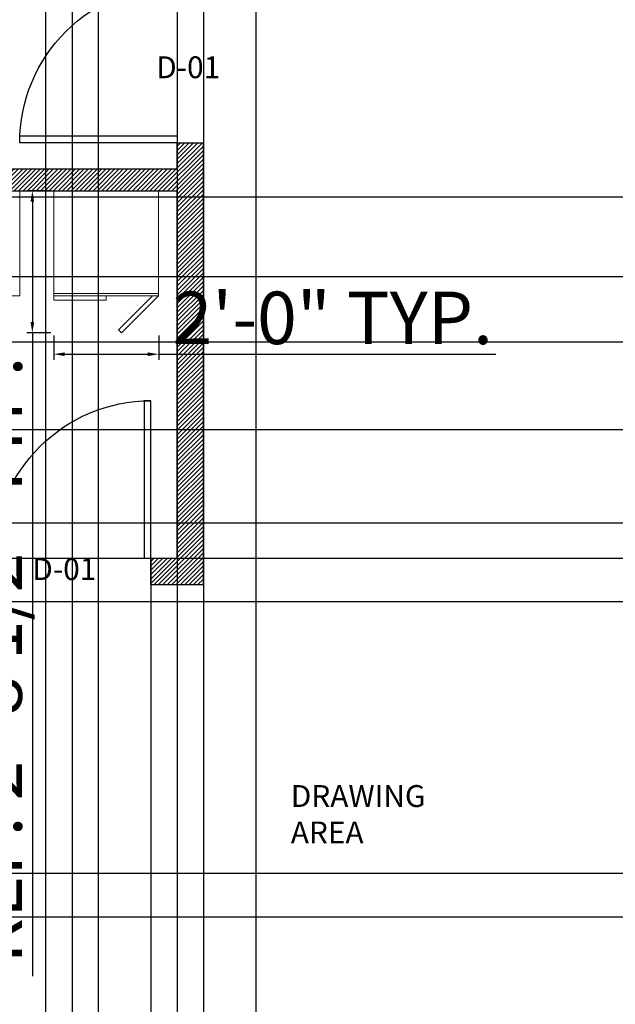
# Model space of a CAD drawing. Units: inches. Extents: x 2386 to 3029, y 792 to 1465.
# Tile 9 of 12: x 2588 to 2724, y 1044 to 1269. Entities that reach past the tile are written whole.
import ezdxf

# ---------------------------------------------------------------- set-up
doc = ezdxf.new("R2010")
doc.units = ezdxf.units.IN
for name, color, linetype, lineweight in [('A-AREA-IDEN', 4, 'Continuous', 25), ('A-DIMS', 1, 'Continuous', 18), ('A-DOOR', 2, 'Continuous', 25), ('A-EQPM', 8, 'Continuous', 18), ('A-FLOR-CASE', 6, 'Continuous', 18), ('A-TEXT', 4, 'Continuous', 25), ('A-WALL-INT', 9, 'Continuous', 30), ('A-WALL-PATT', 9, 'Continuous', 13)]:
    doc.layers.add(name, color=color, linetype=linetype, lineweight=lineweight)
doc.styles.get("Standard").update_dxf_attribs({"font": 'arial.ttf'})
doc.dimstyles.new('ISO-25', dxfattribs={"dimtxt": 12, "dimasz": 2.5, "dimexe": 1.25, "dimexo": 0.625, "dimtad": 1, "dimlunit": 4, "dimtxsty": 'Standard', "dimcen": 2.5, "dimadec": 0, "dimazin": 0, "dimtfac": 1, "dimtmove": 0, "dimatfit": 3, "dimfxl": 1, "dimarcsym": 0})

# ---------------------------------------------------------------- blocks, each defined once
blk = doc.blocks.new('*U13')
for p, q in [((0, 0), (0, 6)), ((40, 0), (40, 6))]:
    blk.add_line(p, q)
blk.add_lwpolyline([(0, 0), (0, -40), (1.75, -40), (1.75, 0)], close=True)
blk.add_arc((0, 0), 40, 270, 0)
blk = doc.blocks.new('*U14')
for p, q in [((-40, 0), (-40, 6)), ((0, 0), (0, 6))]:
    blk.add_line(p, q)
blk.add_lwpolyline([(0, 0), (0, -40), (-1.75, -40), (-1.75, 0)], close=True)
blk.add_arc((0, 0), 40, 180, 270)
blk = doc.blocks.new('REFRIGERATOR-24')
blk.add_line((23.5, 24), (23.5, 0))
for points in [[(24, 0), (0, 0), (0, 24), (24, 24)], [(24, 22.59), (31.78, 14.81), (32.49, 15.51), (24, 24), (24, 0), (25, 0), (25, 12), (24, 12)]]:
    blk.add_lwpolyline(points)
blk = doc.blocks.new('*D52')
at = {"layer": 'A-DIMS', "color": 0, "lineweight": -2, "transparency": 16777216}
for p, q in [((2595.33, 1229.95), (2589.83, 1229.95)), ((2591.08, 1227.45), (2591.08, 1199.96)), ((2595.33, 1197.46), (2589.83, 1197.46)), ((2591.08, 1197.46), (2591.08, 1050.38))]:
    blk.add_line(p, q, dxfattribs=at)
at = {"layer": 'A-DIMS', "color": 0, "transparency": 16777216}
for points in [[(2590.67, 1227.45), (2591.5, 1227.45), (2591.08, 1229.95)], [(2590.67, 1199.96), (2591.5, 1199.96), (2591.08, 1197.46)]]:
    blk.add_solid(points, dxfattribs=at)
at = {"layer": 'Defpoints', "color": 0, "transparency": 16777216}
for p in [(2595.96, 1229.95), (2591.08, 1197.46), (2595.96, 1197.46)]:
    blk.add_point(p, dxfattribs=at)
at = {"layer": 'A-DIMS', "color": 0, "transparency": 16777216, "insert": (2584.25, 1122.67), "char_height": 12, "attachment_point": 5, "rotation": 90}
blk.add_mtext('REF. 2\'-8 1/2" TYP.', dxfattribs=at)
blk = doc.blocks.new('*D53')
at = {"layer": 'A-DIMS', "color": 0, "lineweight": -2, "transparency": 16777216}
for p, q in [((2595.96, 1196.84), (2595.96, 1191.34)), ((2619.96, 1196.84), (2619.96, 1191.34)), ((2598.46, 1192.59), (2617.46, 1192.59)), ((2619.96, 1192.59), (2697.06, 1192.59))]:
    blk.add_line(p, q, dxfattribs=at)
at = {"layer": 'A-DIMS', "color": 0, "transparency": 16777216}
for points in [[(2598.46, 1193.01), (2598.46, 1192.17), (2595.96, 1192.59)], [(2617.46, 1193.01), (2617.46, 1192.17), (2619.96, 1192.59)]]:
    blk.add_solid(points, dxfattribs=at)
at = {"layer": 'Defpoints', "color": 0, "transparency": 16777216}
for p in [(2595.96, 1197.46), (2619.96, 1197.46), (2619.96, 1192.59)]:
    blk.add_point(p, dxfattribs=at)
at = {"layer": 'A-DIMS', "color": 0, "transparency": 16777216, "insert": (2659.76, 1199.34), "char_height": 12, "attachment_point": 5}
blk.add_mtext('2\'-0" TYP.', dxfattribs=at)
blk = doc.blocks.new('*D66')
at = {"layer": 'A-DIMS', "color": 0, "lineweight": -2, "transparency": 16777216}
for p, q in [((2630.19, 1378.32), (2630.19, 808)), ((2642.19, 1378.32), (2642.19, 808)), ((2632.69, 809.25), (2639.69, 809.25)), ((2642.19, 809.25), (2676.71, 809.25))]:
    blk.add_line(p, q, dxfattribs=at)
at = {"layer": 'A-DIMS', "color": 0, "transparency": 16777216}
for points in [[(2632.69, 809.66), (2632.69, 808.83), (2630.19, 809.25)], [(2639.69, 809.66), (2639.69, 808.83), (2642.19, 809.25)]]:
    blk.add_solid(points, dxfattribs=at)
at = {"layer": 'Defpoints', "color": 0, "transparency": 16777216}
for p in [(2630.19, 1378.95), (2642.19, 1378.95), (2642.19, 809.25)]:
    blk.add_point(p, dxfattribs=at)
at = {"layer": 'A-DIMS', "color": 0, "transparency": 16777216, "insert": (2660.7, 816), "char_height": 12, "attachment_point": 5}
blk.add_mtext('1\'-0"', dxfattribs=at)
blk = doc.blocks.new('*D75')
at = {"layer": 'A-DIMS', "color": 0, "lineweight": -2, "transparency": 16777216}
for p, q in [((2929.89, 1195.39), (2929.89, 1229.91)), ((2498.82, 1195.39), (2931.14, 1195.39)), ((2929.89, 1177.89), (2929.89, 1192.89)), ((2498.82, 1175.39), (2931.14, 1175.39))]:
    blk.add_line(p, q, dxfattribs=at)
at = {"layer": 'A-DIMS', "color": 0, "transparency": 16777216}
for points in [[(2929.47, 1192.89), (2930.31, 1192.89), (2929.89, 1195.39)], [(2929.47, 1177.89), (2930.31, 1177.89), (2929.89, 1175.39)]]:
    blk.add_solid(points, dxfattribs=at)
at = {"layer": 'Defpoints', "color": 0, "transparency": 16777216}
for p in [(2498.19, 1195.39), (2929.89, 1195.39), (2498.19, 1175.39)]:
    blk.add_point(p, dxfattribs=at)
at = {"layer": 'A-DIMS', "color": 0, "transparency": 16777216, "insert": (2923.14, 1213.9), "char_height": 12, "attachment_point": 5, "rotation": 90}
blk.add_mtext('1\'-8"', dxfattribs=at)
blk = doc.blocks.new('*D79')
at = {"layer": 'A-DIMS', "color": 0, "lineweight": -2, "transparency": 16777216}
for p, q in [((2929.89, 1073.95), (2929.89, 1118.92)), ((2516.82, 1073.95), (2931.14, 1073.95)), ((2929.89, 1066.45), (2929.89, 1071.45)), ((2516.82, 1063.95), (2931.14, 1063.95))]:
    blk.add_line(p, q, dxfattribs=at)
at = {"layer": 'A-DIMS', "color": 0, "transparency": 16777216}
for points in [[(2929.47, 1071.45), (2930.31, 1071.45), (2929.89, 1073.95)], [(2929.47, 1066.45), (2930.31, 1066.45), (2929.89, 1063.95)]]:
    blk.add_solid(points, dxfattribs=at)
at = {"layer": 'Defpoints', "color": 0, "transparency": 16777216}
for p in [(2516.19, 1073.95), (2929.89, 1073.95), (2516.19, 1063.95)]:
    blk.add_point(p, dxfattribs=at)
at = {"layer": 'A-DIMS', "color": 0, "transparency": 16777216, "insert": (2923.14, 1097.68), "char_height": 12, "attachment_point": 5, "rotation": 90}
blk.add_mtext('0\'-10"', dxfattribs=at)
blk = doc.blocks.new('*D81')
at = {"layer": 'A-DIMS', "color": 0, "lineweight": -2, "transparency": 16777216}
for p, q in [((2432.49, 1153.95), (2432.49, 1188.47)), ((2809.57, 1153.95), (2431.24, 1153.95)), ((2432.49, 1138.45), (2432.49, 1151.45)), ((2809.57, 1135.95), (2431.24, 1135.95))]:
    blk.add_line(p, q, dxfattribs=at)
at = {"layer": 'A-DIMS', "color": 0, "transparency": 16777216}
for points in [[(2432.07, 1151.45), (2432.91, 1151.45), (2432.49, 1153.95)], [(2432.07, 1138.45), (2432.91, 1138.45), (2432.49, 1135.95)]]:
    blk.add_solid(points, dxfattribs=at)
at = {"layer": 'Defpoints', "color": 0, "transparency": 16777216}
for p in [(2432.49, 1153.95), (2810.19, 1153.95), (2810.19, 1135.95)]:
    blk.add_point(p, dxfattribs=at)
at = {"layer": 'A-DIMS', "color": 0, "transparency": 16777216, "insert": (2425.74, 1172.46), "char_height": 12, "attachment_point": 5, "rotation": 90}
blk.add_mtext('1\'-6"', dxfattribs=at)
blk = doc.blocks.new('*D82')
at = {"layer": 'A-DIMS', "color": 0, "lineweight": -2, "transparency": 16777216}
for p, q in [((2600.19, 1306.32), (2600.19, 808)), ((2624.19, 1306.32), (2624.19, 808)), ((2602.69, 809.25), (2621.69, 809.25)), ((2624.19, 809.25), (2660.04, 809.25))]:
    blk.add_line(p, q, dxfattribs=at)
at = {"layer": 'A-DIMS', "color": 0, "transparency": 16777216}
for points in [[(2602.69, 809.66), (2602.69, 808.83), (2600.19, 809.25)], [(2621.69, 809.66), (2621.69, 808.83), (2624.19, 809.25)]]:
    blk.add_solid(points, dxfattribs=at)
at = {"layer": 'Defpoints', "color": 0, "transparency": 16777216}
for p in [(2600.19, 1306.95), (2624.19, 1306.95), (2624.19, 809.25)]:
    blk.add_point(p, dxfattribs=at)
at = {"layer": 'A-DIMS', "color": 0, "transparency": 16777216, "insert": (2643.37, 816), "char_height": 12, "attachment_point": 5}
blk.add_mtext('2\'-0"', dxfattribs=at)
blk = doc.blocks.new('*D87')
at = {"layer": 'A-DIMS', "color": 0, "lineweight": -2, "transparency": 16777216}
for p, q in [((2594.19, 921.57), (2594.19, 1427.9)), ((2606.19, 921.57), (2606.19, 1427.9)), ((2596.69, 1426.65), (2603.69, 1426.65)), ((2606.19, 1426.65), (2640.71, 1426.65))]:
    blk.add_line(p, q, dxfattribs=at)
at = {"layer": 'A-DIMS', "color": 0, "transparency": 16777216}
for points in [[(2596.69, 1427.06), (2596.69, 1426.23), (2594.19, 1426.65)], [(2603.69, 1427.06), (2603.69, 1426.23), (2606.19, 1426.65)]]:
    blk.add_solid(points, dxfattribs=at)
at = {"layer": 'Defpoints', "color": 0, "transparency": 16777216}
for p in [(2606.19, 1426.65), (2594.19, 920.95), (2606.19, 920.95)]:
    blk.add_point(p, dxfattribs=at)
at = {"layer": 'A-DIMS', "color": 0, "transparency": 16777216, "insert": (2624.7, 1433.4), "char_height": 12, "attachment_point": 5}
blk.add_mtext('1\'-0"', dxfattribs=at)
blk = doc.blocks.new('*D92')
at = {"layer": 'A-DIMS', "color": 0, "lineweight": -2, "transparency": 16777216}
for p, q in [((2618.19, 1145.32), (2618.19, 808)), ((2624.19, 1145.32), (2624.19, 808)), ((2615.69, 809.25), (2613.19, 809.25)), ((2618.19, 809.25), (2624.19, 809.25)), ((2626.69, 809.25), (2662.34, 809.25))]:
    blk.add_line(p, q, dxfattribs=at)
at = {"layer": 'A-DIMS', "color": 0, "transparency": 16777216}
for points in [[(2615.69, 809.66), (2615.69, 808.83), (2618.19, 809.25)], [(2626.69, 809.66), (2626.69, 808.83), (2624.19, 809.25)]]:
    blk.add_solid(points, dxfattribs=at)
at = {"layer": 'Defpoints', "color": 0, "transparency": 16777216}
for p in [(2618.19, 1145.95), (2624.19, 1145.95), (2624.19, 809.25)]:
    blk.add_point(p, dxfattribs=at)
at = {"layer": 'A-DIMS', "color": 0, "transparency": 16777216, "insert": (2645.76, 816), "char_height": 12, "attachment_point": 5}
blk.add_mtext('0\'-6"', dxfattribs=at)
blk = doc.blocks.new('*D99')
at = {"layer": 'A-DIMS', "color": 0, "lineweight": -2, "transparency": 16777216}
for p, q in [((2530.41, 1210.29), (2530.41, 808)), ((2563.26, 1210.63), (2563.26, 808)), ((2532.91, 809.25), (2560.76, 809.25)), ((2563.26, 809.25), (2599.11, 809.25))]:
    blk.add_line(p, q, dxfattribs=at)
at = {"layer": 'A-DIMS', "color": 0, "transparency": 16777216}
for points in [[(2532.91, 809.66), (2532.91, 808.83), (2530.41, 809.25)], [(2560.76, 809.66), (2560.76, 808.83), (2563.26, 809.25)]]:
    blk.add_solid(points, dxfattribs=at)
at = {"layer": 'Defpoints', "color": 0, "transparency": 16777216}
for p in [(2563.26, 1211.26), (2530.41, 1210.91), (2563.26, 809.25)]:
    blk.add_point(p, dxfattribs=at)
at = {"layer": 'A-DIMS', "color": 0, "transparency": 16777216, "insert": (2582.43, 816), "char_height": 12, "attachment_point": 5}
blk.add_mtext('2\'-9"', dxfattribs=at)
blk = doc.blocks.new('*D100')
at = {"layer": 'A-DIMS', "color": 0, "lineweight": -2, "transparency": 16777216}
for p, q in [((2562.86, 1228.59), (2931.14, 1228.59)), ((2929.89, 1226.09), (2929.89, 1212.84)), ((2563.05, 1210.34), (2931.14, 1210.34)), ((2929.89, 1210.34), (2929.89, 1147.86))]:
    blk.add_line(p, q, dxfattribs=at)
at = {"layer": 'A-DIMS', "color": 0, "transparency": 16777216}
for points in [[(2929.47, 1226.09), (2930.31, 1226.09), (2929.89, 1228.59)], [(2929.47, 1212.84), (2930.31, 1212.84), (2929.89, 1210.34)]]:
    blk.add_solid(points, dxfattribs=at)
at = {"layer": 'Defpoints', "color": 0, "transparency": 16777216}
for p in [(2562.24, 1228.59), (2562.43, 1210.34), (2929.89, 1210.34)]:
    blk.add_point(p, dxfattribs=at)
at = {"layer": 'A-DIMS', "color": 0, "transparency": 16777216, "insert": (2923.06, 1177.85), "char_height": 12, "attachment_point": 5, "rotation": 90}
blk.add_mtext('1\'-6 1/2"', dxfattribs=at)
blk = doc.blocks.new('*D101')
at = {"layer": 'A-DIMS', "color": 0, "lineweight": -2, "transparency": 16777216}
for p, q in [((2929.89, 1175.39), (2929.89, 1239.21)), ((2480.82, 1175.39), (2931.14, 1175.39)), ((2929.89, 1148.45), (2929.89, 1172.89)), ((2480.82, 1145.95), (2931.14, 1145.95))]:
    blk.add_line(p, q, dxfattribs=at)
at = {"layer": 'A-DIMS', "color": 0, "transparency": 16777216}
for points in [[(2929.47, 1172.89), (2930.31, 1172.89), (2929.89, 1175.39)], [(2929.47, 1148.45), (2930.31, 1148.45), (2929.89, 1145.95)]]:
    blk.add_solid(points, dxfattribs=at)
at = {"layer": 'Defpoints', "color": 0, "transparency": 16777216}
for p in [(2480.19, 1175.39), (2929.89, 1175.39), (2480.19, 1145.95)]:
    blk.add_point(p, dxfattribs=at)
at = {"layer": 'A-DIMS', "color": 0, "transparency": 16777216, "insert": (2923.06, 1208.55), "char_height": 12, "attachment_point": 5, "rotation": 90}
blk.add_mtext('2\'-5 1/2"', dxfattribs=at)

msp = doc.modelspace()

# ---------------------------------------------------------------- hatches: boundary and pattern name
at = {"layer": 'A-WALL-PATT'}
h = msp.add_hatch(dxfattribs=at)
h.set_pattern_fill('JIS_WOOD', color=256)
h.paths.add_polyline_path([(2624.19, 1229.948), (2624.19, 1145.948), (2618.19, 1145.948), (2618.19, 1140.548), (2618.19, 1139.948), (2630.19, 1139.948), (2630.19, 1240.948), (2624.19, 1240.948), (2624.19, 1234.948), (2480.19, 1234.948), (2480.19, 1229.948)])
h.paths.add_polyline_path([(2582.19, 1139.948), (2582.19, 1145.948), (2480.19, 1145.948), (2480.19, 1139.948)], flags=17)
h.paths.add_polyline_path([(2480.19, 1007.948), (2480.19, 1001.948), (2546.19, 1001.948), (2546.19, 1007.348), (2546.19, 1007.948)])
h.paths.add_polyline_path([(2594.19, 1007.948), (2582.19, 1007.948), (2582.19, 1001.948), (2588.19, 1001.948), (2588.19, 856.948), (2594.19, 856.948), (2594.19, 914.948), (2606.19, 914.948), (2606.19, 920.948), (2594.19, 920.948)])
h.paths.add_polyline_path([(2738.19, 1015.948), (2882.19, 1015.948), (2882.19, 1021.948), (2738.19, 1021.948), (2738.19, 1111.948), (2732.19, 1111.948), (2732.19, 920.948), (2720.19, 920.948), (2720.19, 914.948), (2732.19, 914.948), (2732.19, 856.948), (2738.19, 856.948)])
h.paths.add_polyline_path([(2660.19, 914.948), (2660.19, 920.948), (2648.19, 920.948), (2648.19, 914.948)])
h.paths.add_polyline_path([(2738.19, 1159.948), (2738.19, 1165.948), (2737.59, 1165.948), (2732.19, 1165.948), (2732.19, 1147.948), (2737.59, 1147.948), (2738.19, 1147.948), (2738.19, 1153.948), (2882.19, 1153.948), (2882.19, 1159.948)])
h.paths.add_polyline_path([(2732.19, 1201.948), (2738.19, 1201.948), (2738.19, 1303.948), (2774.19, 1303.948), (2774.19, 1308.948), (2768.19, 1308.948), (2768.19, 1378.948), (2762.19, 1378.948), (2762.19, 1308.948), (2726.19, 1308.948), (2726.19, 1303.948), (2732.19, 1303.948)])
h.paths.add_polyline_path([(2696.19, 1303.948), (2696.19, 1308.948), (2630.19, 1308.948), (2630.19, 1378.948), (2624.19, 1378.948), (2624.19, 1276.948), (2630.19, 1276.948), (2630.19, 1303.948)])

# ---------------------------------------------------------------- linework, layer by layer
at = {"layer": 'A-FLOR-CASE'}
msp.add_lwpolyline([(2504.19, 1145.948), (2504.19, 1205.948), (2588.19, 1205.948), (2588.19, 1229.948)], dxfattribs=at)
at = {"layer": 'A-WALL-INT'}
for p, q in [((2624.19, 1234.948), (2624.19, 1240.948)), ((2624.19, 1240.948), (2630.19, 1240.948)), ((2630.19, 1139.948), (2630.19, 1240.948)), ((2480.19, 1234.948), (2624.19, 1234.948)), ((2480.19, 1229.948), (2624.19, 1229.948)), ((2624.19, 1145.948), (2624.19, 1229.948)), ((2618.19, 1139.948), (2618.19, 1145.948)), ((2618.19, 1145.948), (2624.19, 1145.948)), ((2618.19, 1139.948), (2630.19, 1139.948))]:
    msp.add_line(p, q, dxfattribs=at)

# ---------------------------------------------------------------- block references
at = {"layer": 'A-DOOR', "xscale": -0.9, "yscale": 0.9, "zscale": 0.9}
for name, p, rotation in [('*U13', (2624.19, 1240.948), 270), ('*U14', (2618.19, 1145.948), 180)]:
    msp.add_blockref(name, p, dxfattribs=dict(at, rotation=rotation))
at = {"layer": 'A-EQPM', "rotation": 269.9999999999993}
msp.add_blockref('REFRIGERATOR-24', (2595.956, 1229.948), dxfattribs=at)

# ---------------------------------------------------------------- texts
at = {"layer": 'A-AREA-IDEN', "insert": (2650.166, 1094.069), "char_height": 5, "attachment_point": 1}
msp.add_mtext_dynamic_manual_height_columns('DRAWING    AREA', width=38.22215, gutter_width=12.5, heights=[0], dxfattribs=at)
at = {"layer": 'A-TEXT', "char_height": 5, "attachment_point": 1}
for insert in [(2619.392, 1260.698), (2591.074, 1145.947)]:
    msp.add_mtext_dynamic_manual_height_columns('D-01', width=38.22215, gutter_width=12.5, heights=[0], dxfattribs=dict(at, insert=insert))

# ---------------------------------------------------------------- dimensions: what is measured, and where the dimension line sits
at = {"layer": 'A-DIMS'}
for base, p1, p2, picture, middle in [((2606.19, 1426.648), (2594.19, 920.948), (2606.19, 920.948), '*D87', (2624.7, 1433.4)), ((2642.19, 809.248), (2630.19, 1378.948), (2642.19, 1378.948), '*D66', (2660.7, 816)), ((2624.19, 809.248), (2600.19, 1306.948), (2624.19, 1306.948), '*D82', (2643.367, 816)), ((2563.257, 809.248), (2530.413, 1210.915), (2563.257, 1211.257), '*D99', (2582.434, 816)), ((2624.19, 809.248), (2618.19, 1145.948), (2624.19, 1145.948), '*D92', (2645.765, 816))]:
    dim = msp.add_linear_dim(base=base, p1=p1, p2=p2, dimstyle='ISO-25', override={"dimdec": 1, "dimlfac": 1, "dimrnd": 0, "dimzin": 1, "dimdsep": 46, "dimlunit": 4, "dimfrac": 2}, dxfattribs=at)
    dim.commit()
    dim.dimension.update_dxf_attribs({"geometry": picture, "text_midpoint": middle})
for base, p1, p2, picture, middle in [((2929.89, 1175.392), (2480.19, 1145.948), (2480.19, 1175.392), '*D101', (2923.06, 1208.55)), ((2929.89, 1195.392), (2498.19, 1175.392), (2498.19, 1195.392), '*D75', (2923.138, 1213.902)), ((2929.89, 1210.342), (2562.236, 1228.595), (2562.425, 1210.342), '*D100', (2923.06, 1177.852)), ((2432.49, 1153.948), (2810.19, 1135.948), (2810.19, 1153.948), '*D81', (2425.738, 1172.458)), ((2929.89, 1073.948), (2516.19, 1063.948), (2516.19, 1073.948), '*D79', (2923.138, 1097.684))]:
    dim = msp.add_linear_dim(base=base, p1=p1, p2=p2, angle=90, dimstyle='ISO-25', override={"dimdec": 1, "dimlfac": 1, "dimrnd": 0, "dimzin": 1, "dimdsep": 46, "dimlunit": 4, "dimfrac": 2}, dxfattribs=at)
    dim.commit()
    dim.dimension.update_dxf_attribs({"geometry": picture, "text_midpoint": middle})
dim = msp.add_linear_dim(base=(2591.083, 1197.463), p1=(2595.956, 1229.948), p2=(2595.956, 1197.463), angle=270, text='REF. <> TYP.', dimstyle='ISO-25', override={"dimdec": 1, "dimlfac": 1, "dimrnd": 0, "dimzin": 1, "dimdsep": 46, "dimlunit": 4, "dimfrac": 2}, dxfattribs=at)
dim.commit()
dim.dimension.update_dxf_attribs({"geometry": '*D52', "text_midpoint": (2584.253, 1122.673)})
dim = msp.add_linear_dim(base=(2619.956, 1192.59), p1=(2595.956, 1197.463), p2=(2619.956, 1197.463), text='<> TYP.', dimstyle='ISO-25', override={"dimdec": 1, "dimlfac": 1, "dimrnd": 0, "dimzin": 1, "dimdsep": 46, "dimlunit": 4, "dimfrac": 2}, dxfattribs=at)
dim.commit()
dim.dimension.update_dxf_attribs({"geometry": '*D53', "text_midpoint": (2659.756, 1199.342)})

doc.saveas('drawing.dxf')
